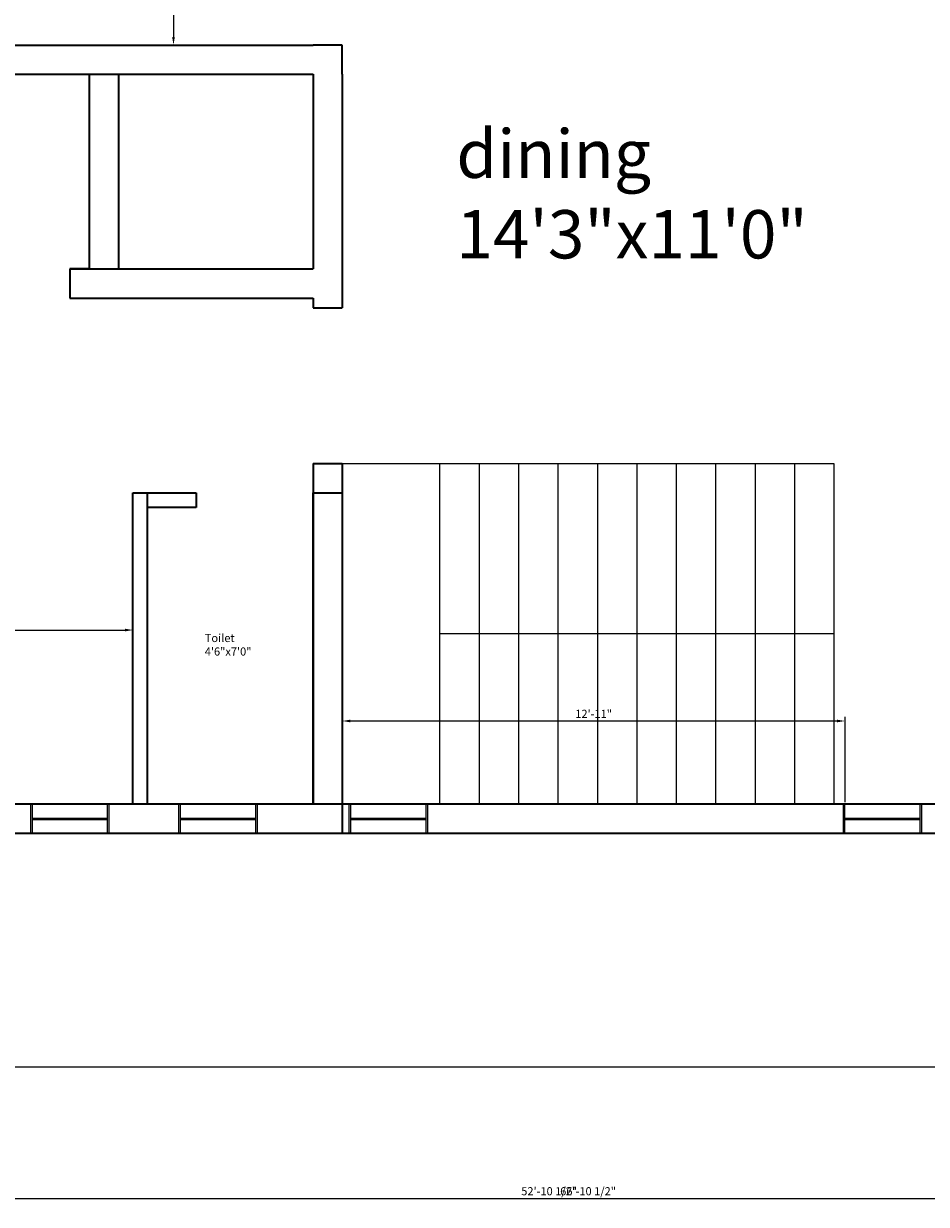
# Model space of a CAD drawing. Units: inches. Extents: x 250205121 to 250208111, y 89832590 to 89833271.
# Tile 6 of 14: x 250206445 to 250206724, y 89832600 to 89832964. Entities that reach past the tile are written whole.
import ezdxf

# ---------------------------------------------------------------- set-up
doc = ezdxf.new("R2010")
doc.units = ezdxf.units.IN
for name, color, linetype, lineweight in [('A-AREA-IDEN', 4, 'Continuous', 18), ('A-FLOR-STRS', 7, 'Continuous', 25), ('A-WALL', 7, 'Continuous', 35), ('C-PROP', 8, 'Continuous', 25), ('dimensions', 2, 'Continuous', 18), ('window', 4, 'Continuous', 18)]:
    doc.layers.add(name, color=color, linetype=linetype, lineweight=lineweight)
doc.styles.get("Standard").update_dxf_attribs({"font": 'arial.ttf'})
doc.dimstyles.new('ISO-25', dxfattribs={"dimtxt": 2.5, "dimasz": 2.5, "dimexe": 1.25, "dimexo": 0.625, "dimtad": 1, "dimlunit": 4, "dimtxsty": 'Standard', "dimcen": 2.5, "dimadec": 0, "dimazin": 0, "dimtfac": 1, "dimtmove": 0, "dimatfit": 3, "dimfxl": 1, "dimarcsym": 0})

# ---------------------------------------------------------------- blocks, each defined once
blk = doc.blocks.new('*D10')
at = {"layer": 'Defpoints', "color": 0, "transparency": 16777216}
for p in [(250206514.09, 89833134.33), (250206491.68, 89832957.33), (250206514.09, 89832957.33)]:
    blk.add_point(p, dxfattribs=at)
at = {"layer": 'dimensions', "color": 0, "lineweight": -2, "transparency": 16777216}
for p, q in [((250206513.46, 89833134.33), (250206490.43, 89833134.33)), ((250206491.68, 89833131.83), (250206491.68, 89832959.83)), ((250206513.46, 89832957.33), (250206490.43, 89832957.33))]:
    blk.add_line(p, q, dxfattribs=at)
at = {"layer": 'dimensions', "color": 0, "transparency": 16777216}
for points in [[(250206491.26, 89833131.83), (250206492.1, 89833131.83), (250206491.68, 89833134.33)], [(250206491.26, 89832959.83), (250206492.1, 89832959.83), (250206491.68, 89832957.33)]]:
    blk.add_solid(points, dxfattribs=at)
at = {"layer": 'dimensions', "color": 0, "transparency": 16777216, "insert": (250206489.78, 89833045.83), "char_height": 2.5, "attachment_point": 5, "rotation": 90}
blk.add_mtext('14\'-9"', dxfattribs=at)
blk = doc.blocks.new('*D14')
at = {"layer": 'Defpoints', "color": 0, "transparency": 16777216}
for p in [(250206479.19, 89832777.03), (250206299.19, 89832769.11), (250206479.19, 89832769.11)]:
    blk.add_point(p, dxfattribs=at)
at = {"layer": 'dimensions', "color": 0, "lineweight": -2, "transparency": 16777216}
for p, q in [((250206299.19, 89832769.73), (250206299.19, 89832778.28)), ((250206301.69, 89832777.03), (250206476.69, 89832777.03)), ((250206479.19, 89832769.73), (250206479.19, 89832778.28))]:
    blk.add_line(p, q, dxfattribs=at)
at = {"layer": 'dimensions', "color": 0, "transparency": 16777216}
for points in [[(250206301.69, 89832777.44), (250206301.69, 89832776.61), (250206299.19, 89832777.03)], [(250206476.69, 89832777.44), (250206476.69, 89832776.61), (250206479.19, 89832777.03)]]:
    blk.add_solid(points, dxfattribs=at)
at = {"layer": 'dimensions', "color": 0, "transparency": 16777216, "insert": (250206389.19, 89832778.93), "char_height": 2.5, "attachment_point": 5}
blk.add_mtext("15'", dxfattribs=at)
blk = doc.blocks.new('*D16')
at = {"layer": 'Defpoints', "color": 0, "transparency": 16777216}
for p in [(250206698.61, 89832749), (250206543.69, 89832723.33), (250206698.61, 89832723.33)]:
    blk.add_point(p, dxfattribs=at)
at = {"layer": 'dimensions', "color": 0, "lineweight": -2, "transparency": 16777216}
for p, q in [((250206543.69, 89832723.95), (250206543.69, 89832750.25)), ((250206546.19, 89832749), (250206696.11, 89832749)), ((250206698.61, 89832723.95), (250206698.61, 89832750.25))]:
    blk.add_line(p, q, dxfattribs=at)
at = {"layer": 'dimensions', "color": 0, "transparency": 16777216}
for points in [[(250206546.19, 89832749.41), (250206546.19, 89832748.58), (250206543.69, 89832749)], [(250206696.11, 89832749.41), (250206696.11, 89832748.58), (250206698.61, 89832749)]]:
    blk.add_solid(points, dxfattribs=at)
at = {"layer": 'dimensions', "color": 0, "transparency": 16777216, "insert": (250206621.15, 89832750.88), "char_height": 2.5, "attachment_point": 5}
blk.add_mtext('12\'-11"', dxfattribs=at)
blk = doc.blocks.new('WIN-24IN')
for p, q in [((0, 0), (0, 24.08)), ((0, 24.08), (9, 24.08)), ((0, 23.58), (9, 23.58)), ((4.3, 23.58), (4.3, 0.5)), ((4.7, 23.58), (4.7, 0.5)), ((9, 24.08), (9, 0)), ((9, 0.5), (0, 0.5)), ((9, 0), (0, 0))]:
    blk.add_line(p, q)
blk = doc.blocks.new('STAIR-CENTRAL')
for p, q in [((0, 105), (30, 105)), ((30, 105), (30, 0)), ((30, 105), (151.5, 105)), ((42.15, 105), (42.15, 0)), ((54.3, 105), (54.3, 0)), ((66.45, 105), (66.45, 0)), ((78.6, 105), (78.6, 0)), ((90.75, 105), (90.75, 0)), ((102.9, 105), (102.9, 0)), ((115.05, 105), (115.05, 0)), ((127.2, 105), (127.2, 0)), ((139.35, 105), (139.35, 0)), ((151.5, 105), (151.5, 0)), ((151.5, 105), (151.5, 0)), ((151.5, 52.5), (30, 52.5)), ((0, 0), (6, 0)), ((6, 0), (30, 0)), ((30, 0), (151.5, 0)), ((151.5, 0), (175.5, 0)), ((175.5, 0), (181.5, 0))]:
    blk.add_line(p, q)
blk = doc.blocks.new('*D54')
at = {"layer": 'Defpoints', "color": 0, "transparency": 16777216}
for p in [(250206218.19, 89832642.33), (250207020.69, 89832642.33), (250207020.69, 89832601.83)]:
    blk.add_point(p, dxfattribs=at)
at = {"layer": 'dimensions', "color": 0, "lineweight": -2, "transparency": 16777216}
for p, q in [((250206218.19, 89832641.7), (250206218.19, 89832600.58)), ((250207020.69, 89832641.7), (250207020.69, 89832600.58)), ((250206220.69, 89832601.83), (250207018.19, 89832601.83))]:
    blk.add_line(p, q, dxfattribs=at)
at = {"layer": 'dimensions', "color": 0, "transparency": 16777216}
for points in [[(250206220.69, 89832602.24), (250206220.69, 89832601.41), (250206218.19, 89832601.83)], [(250207018.19, 89832602.24), (250207018.19, 89832601.41), (250207020.69, 89832601.83)]]:
    blk.add_solid(points, dxfattribs=at)
at = {"layer": 'dimensions', "color": 0, "transparency": 16777216, "insert": (250206619.44, 89832603.75), "char_height": 2.5, "attachment_point": 5}
blk.add_mtext('66\'-10 1/2"', dxfattribs=at)
blk = doc.blocks.new('*D61')
at = {"layer": 'Defpoints', "color": 0, "transparency": 16777216}
for p in [(250206290.19, 89832714.33), (250206924.69, 89832714.33), (250206924.69, 89832601.83)]:
    blk.add_point(p, dxfattribs=at)
at = {"layer": 'dimensions', "color": 0, "lineweight": -2, "transparency": 16777216}
for p, q in [((250206290.19, 89832713.7), (250206290.19, 89832600.58)), ((250206924.69, 89832713.7), (250206924.69, 89832600.58)), ((250206292.69, 89832601.83), (250206922.19, 89832601.83))]:
    blk.add_line(p, q, dxfattribs=at)
at = {"layer": 'dimensions', "color": 0, "transparency": 16777216}
for points in [[(250206292.69, 89832602.24), (250206292.69, 89832601.41), (250206290.19, 89832601.83)], [(250206922.19, 89832602.24), (250206922.19, 89832601.41), (250206924.69, 89832601.83)]]:
    blk.add_solid(points, dxfattribs=at)
at = {"layer": 'dimensions', "color": 0, "transparency": 16777216, "insert": (250206607.44, 89832603.75), "char_height": 2.5, "attachment_point": 5}
blk.add_mtext('52\'-10 1/2"', dxfattribs=at)

msp = doc.modelspace()

# ---------------------------------------------------------------- linework, layer by layer
at = {"layer": 'A-WALL'}
for p, q in [((250206299.187, 89832957.328), (250206534.687, 89832957.328)), ((250206543.687, 89832957.328), (250206534.687, 89832957.328)), ((250206543.687, 89832948.328), (250206543.687, 89832957.328)), ((250206290.187, 89832948.328), (250206534.687, 89832948.328)), ((250206465.687, 89832948.328), (250206465.687, 89832888.328)), ((250206474.687, 89832948.328), (250206474.687, 89832888.328)), ((250206534.687, 89832948.328), (250206534.687, 89832888.328)), ((250206543.687, 89832948.328), (250206543.687, 89832879.328)), ((250206459.687, 89832888.328), (250206534.687, 89832888.328)), ((250206465.687, 89832888.328), (250206459.687, 89832888.328)), ((250206459.687, 89832888.328), (250206459.687, 89832879.328)), ((250206459.687, 89832879.328), (250206534.687, 89832879.328)), ((250206534.687, 89832879.328), (250206534.687, 89832876.328)), ((250206543.687, 89832879.328), (250206543.687, 89832876.328)), ((250206534.687, 89832876.328), (250206543.687, 89832876.328)), ((250206534.687, 89832828.328), (250206534.687, 89832723.328)), ((250206534.687, 89832828.328), (250206543.687, 89832828.328)), ((250206543.687, 89832828.328), (250206543.687, 89832723.328)), ((250206479.187, 89832801.328), (250206479.187, 89832819.328)), ((250206479.187, 89832819.328), (250206483.687, 89832819.328)), ((250206483.687, 89832801.328), (250206483.687, 89832819.328)), ((250206483.687, 89832819.328), (250206498.687, 89832819.328)), ((250206498.687, 89832819.328), (250206498.687, 89832814.828)), ((250206534.687, 89832801.328), (250206534.687, 89832819.328)), ((250206534.687, 89832819.328), (250206543.687, 89832819.328)), ((250206498.687, 89832814.828), (250206483.687, 89832814.828)), ((250206479.187, 89832723.328), (250206479.187, 89832801.328)), ((250206483.687, 89832723.328), (250206483.687, 89832801.328)), ((250206534.687, 89832741.328), (250206534.687, 89832801.328)), ((250206534.687, 89832723.328), (250206534.687, 89832741.328)), ((250206840.687, 89832723.328), (250206299.187, 89832723.328)), ((250206543.687, 89832723.328), (250206543.687, 89832714.328)), ((250206840.687, 89832714.328), (250206307.687, 89832714.328))]:
    msp.add_line(p, q, dxfattribs=at)
at = {"layer": 'C-PROP'}
for p, q in [((250206543.687, 89832642.328), (250206218.187, 89832642.328)), ((250207020.687, 89832642.328), (250206543.687, 89832642.328))]:
    msp.add_line(p, q, dxfattribs=at)

# ---------------------------------------------------------------- block references
at = {"layer": 'A-FLOR-STRS'}
msp.add_blockref('STAIR-CENTRAL', (250206543.687, 89832723.328), dxfattribs=at)
at = {"layer": 'window'}
for p, rotation in [((250206471.77, 89832714.328), 90.00000015586075), ((250206517.448, 89832714.328), 90.00000024888803), ((250206569.937, 89832714.328), 90.00000015586075), ((250206722.187, 89832714.328), 90.0000002954017)]:
    msp.add_blockref('WIN-24IN', p, dxfattribs=dict(at, rotation=rotation))

# ---------------------------------------------------------------- texts
at = {"layer": 'A-AREA-IDEN', "attachment_point": 1}
for s, width, gutter_width, insert, char_height in [('dining\\P14\'3"x11\'0"', 23.63705, 74.43, (250206578.834, 89832931.255), 14.88606), ('Toilet\\P4\'6"x7\'0"', 2.73747, 12.5, (250206501.316, 89832775.828), 2.5)]:
    msp.add_mtext_dynamic_manual_height_columns(s, width=width, gutter_width=gutter_width, heights=[0], dxfattribs=dict(at, insert=insert, char_height=char_height))

# ---------------------------------------------------------------- dimensions: what is measured, and where the dimension line sits
at = {"layer": 'dimensions'}
dim = msp.add_linear_dim(base=(250206491.68, 89832957.328), p1=(250206514.089, 89833134.328), p2=(250206514.089, 89832957.328), angle=90, dimstyle='ISO-25', override={"dimclrd": 0, "dimclre": 0, "dimclrt": 0}, dxfattribs=at)
dim.commit()
dim.dimension.update_dxf_attribs({"geometry": '*D10', "text_midpoint": (250206489.778, 89833045.828)})
for base, p1, p2, override, picture, middle in [((250206479.187, 89832777.026), (250206299.187, 89832769.105), (250206479.187, 89832769.105), {"dimclrd": 0, "dimclre": 0, "dimclrt": 0}, '*D14', (250206389.187, 89832778.928)), ((250206698.608, 89832748.997), (250206543.687, 89832723.328), (250206698.608, 89832723.328), {"dimclrd": 0, "dimclre": 0, "dimclrt": 0}, '*D16', (250206621.148, 89832750.877)), ((250206924.687, 89832601.828), (250206290.187, 89832714.328), (250206924.687, 89832714.328), {"dimdec": 1, "dimlfac": 1, "dimrnd": 0, "dimzin": 1, "dimdsep": 46, "dimlunit": 4, "dimfrac": 2}, '*D61', (250206607.437, 89832603.746)), ((250207020.687, 89832601.828), (250206218.187, 89832642.328), (250207020.687, 89832642.328), {"dimdec": 1, "dimlfac": 1, "dimrnd": 0, "dimzin": 1, "dimdsep": 46, "dimlunit": 4, "dimfrac": 2}, '*D54', (250206619.437, 89832603.746))]:
    dim = msp.add_linear_dim(base=base, p1=p1, p2=p2, dimstyle='ISO-25', override=override, dxfattribs=at)
    dim.commit()
    dim.dimension.update_dxf_attribs({"geometry": picture, "text_midpoint": middle})

doc.saveas('drawing.dxf')
